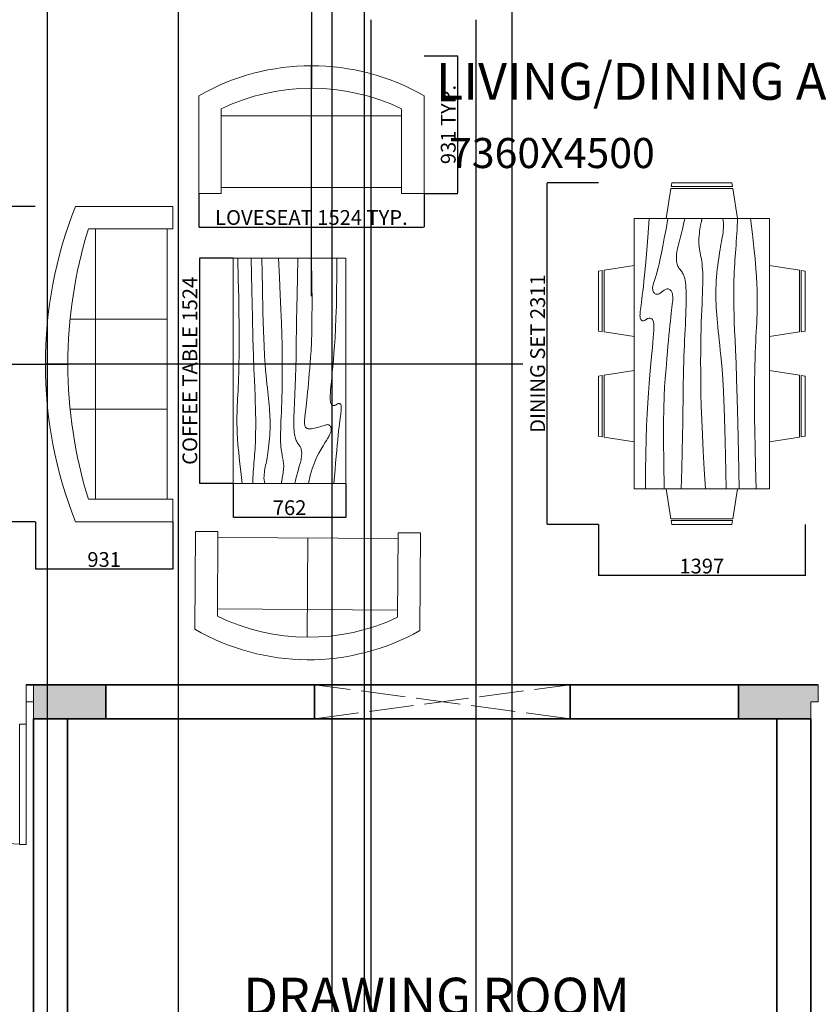
# Model space of a CAD drawing. Units: millimetres. Extents: x -17016 to 4866, y -18325 to 4338.
# Tile 3 of 5: x -8803 to -3399, y -9462 to -2799. Entities that reach past the tile are written whole.
import ezdxf

# ---------------------------------------------------------------- set-up
doc = ezdxf.new("R2010")
doc.units = ezdxf.units.MM
doc.header["$LTSCALE"] = 5
doc.linetypes.add('ACAD_ISO02W100', pattern=[15, 12, -3])
for name, color, linetype, lineweight in [('A-ANNO-DIMS', 2, 'Continuous', 18), ('A-AREA-IDEN', 7, 'Continuous', 25), ('A-COLS', 7, 'Continuous', 35), ('A-COLS-PATT', 252, 'Continuous', 13), ('A-DOOR', 3, 'Continuous', 18), ('A-FURN', 8, 'Continuous', 18), ('A-WALL', 7, 'Continuous', 35), ('A-WALL-OVHD', 8, 'ACAD_ISO02W100', 13)]:
    doc.layers.add(name, color=color, linetype=linetype, lineweight=lineweight)
doc.styles.get("Standard").update_dxf_attribs({"font": 'arial.ttf'})
doc.dimstyles.new('Copy of ISO-25', dxfattribs={"dimtxt": 100, "dimasz": 2.5, "dimexe": 1.25, "dimexo": 0.625, "dimtad": 1, "dimdec": 0, "dimtxsty": 'Standard', "dimcen": 2.5, "dimadec": 0, "dimazin": 0, "dimtfac": 1, "dimtdec": 0, "dimtmove": 0, "dimatfit": 3, "dimfxl": 1, "dimarcsym": 0})

# ---------------------------------------------------------------- blocks, each defined once
blk = doc.blocks.new('Sofa - Roundback 7 ft.')
for p, q in [((-12.00002, -32.4421), (-12.00003, -6.5971)), ((11.99997, -32.4421), (11.99998, -6.5971)), ((-36.000027, -34), (-36.000027, -11.4696)), ((35.99998, -34), (35.99998, -11.4696)), ((-35.999844, -13.3819), (35.9998, -13.3819)), ((-36.000027, -32.4421), (35.99998, -32.4421))]:
    blk.add_line(p, q)
for points in [[(-36.000027, -34), (-42.000027, -34), (-42.000027, -8)], [(41.99998, -8), (41.99998, -34), (35.99998, -34)]]:
    blk.add_lwpolyline(points)
for centre, radius, start, end in [((0, -114.25), 114.25, 68.43141, 111.5686), ((-0.00001, -127.1968), 121.1968, 72.72033, 107.2797)]:
    blk.add_arc(centre, radius, start, end)
blk = doc.blocks.new('Sofa - Roundback Loveseat 5 ft.')
for p, q in [((0, -32.44198), (0, -5.99998)), ((-24, -33.99998), (-24, -11.46958)), ((24.00004, -33.99998), (24.00004, -11.46958)), ((-23.9998, -13.38178), (23.99986, -13.38178)), ((-24, -32.44198), (24.00004, -32.44198))]:
    blk.add_line(p, q)
for points in [[(-24, -33.99998), (-30, -33.99998), (-30, -7.99998)], [(30.00004, -7.99998), (30.00004, -33.99998), (24.00004, -33.99998)]]:
    blk.add_lwpolyline(points)
for centre, radius, start, end in [((0, -60.24998), 60.24998, 60.13715, 119.8628), ((0, -61.38438), 55.38444, 64.32083, 115.6792)]:
    blk.add_arc(centre, radius, start, end)
blk = doc.blocks.new('Table - Rectangular Woodgrain 60 x 30 in.')
for p, q in [((0, 0), (0, -30)), ((60, 0), (0, 0)), ((60, -30), (60, 0)), ((0, -30), (60, -30))]:
    blk.add_line(p, q)
for points in [[(0, -2.4), (4.8155, -2.418), (9.0302, -2.4688), (12.709, -2.5477), (15.9167, -2.65), (18.7181, -2.7711), (21.1781, -2.9063), (23.3616, -3.0508), (25.3333, -3.2), (27.1477, -3.3495), (28.8172, -3.4958), (30.3437, -3.636), (31.7291, -3.7667), (32.9756, -3.8849), (34.0849, -3.9875), (35.059, -4.0714), (35.9, -4.1334), (36.6114, -4.1711), (37.2041, -4.1854), (37.6906, -4.1779), (38.0833, -4.15), (38.3948, -4.1034), (38.6375, -4.0396), (38.8239, -3.9602), (38.9666, -3.8667), (39.0764, -3.7608), (39.1573, -3.6448), (39.2116, -3.521), (39.2416, -3.3917), (39.2498, -3.2593), (39.2385, -3.1261), (39.21, -2.9944), (39.1666, -2.8667), (39.111, -2.7447), (39.0468, -2.6281), (38.978, -2.5163), (38.9083, -2.4083), (38.8418, -2.3035), (38.7823, -2.201), (38.7337, -2.1001), (38.7, -2), (38.6844, -1.9003), (38.6875, -1.8021), (38.7094, -1.707), (38.75, -1.6167), (38.8094, -1.5326), (38.8875, -1.4563), (38.9844, -1.3893), (39.1, -1.3333), (39.2351, -1.2896), (39.3937, -1.2583), (39.5804, -1.2396), (39.8, -1.2333), (40.057, -1.2396), (40.3562, -1.2583), (40.7023, -1.2896), (41.1, -1.3333), (41.5547, -1.3895), (42.0755, -1.4573), (42.6721, -1.5361), (43.3542, -1.625), (44.1316, -1.7233), (45.014, -1.8302), (46.0114, -1.9449), (47.1333, -2.0667), (48.3862, -2.1947), (49.7625, -2.3281), (51.2513, -2.4663), (52.8416, -2.6083), (54.5226, -2.7535), (56.2833, -2.9011), (58.1127, -3.0501), (60, -3.2)], [(0, -9.2), (6.5759, -9.0858), (11.9385, -9.0365), (16.2527, -9.0418), (19.6833, -9.0917), (22.3952, -9.1759), (24.5531, -9.2844), (26.322, -9.4069), (27.8666, -9.5333), (29.3241, -9.6553), (30.7203, -9.7719), (32.0532, -9.8837), (33.3208, -9.9917), (34.5213, -10.0965), (35.6526, -10.199), (36.7128, -10.2999), (37.7, -10.4), (38.6129, -10.4996), (39.4531, -10.5969), (40.223, -10.6895), (40.925, -10.775), (41.5613, -10.8512), (42.1344, -10.9156), (42.6465, -10.966), (43.1, -11), (43.4976, -11.0158), (43.8437, -11.0136), (44.143, -10.9942), (44.4, -10.9583), (44.6195, -10.9069), (44.8062, -10.8406), (44.9648, -10.7603), (45.1, -10.6667), (45.2155, -10.5598), (45.3114, -10.4365), (45.3871, -10.2929), (45.4416, -10.125), (45.4743, -9.929), (45.4844, -9.7011), (45.4709, -9.4371), (45.4333, -9.1333), (45.3716, -8.7883), (45.2896, -8.4104), (45.1919, -8.0107), (45.0833, -7.6), (44.9685, -7.1893), (44.8521, -6.7896), (44.7388, -6.4117), (44.6333, -6.0667), (44.54, -5.7628), (44.4614, -5.4979), (44.4001, -5.2675), (44.3583, -5.0667), (44.3384, -4.8909), (44.3427, -4.7354), (44.3736, -4.5956), (44.4333, -4.4667), (44.5236, -4.3453), (44.6427, -4.2333), (44.7884, -4.1339), (44.9583, -4.05), (45.1501, -3.9849), (45.3614, -3.9417), (45.59, -3.9234), (45.8333, -3.9333), (46.0915, -3.9749), (46.3734, -4.0531), (46.6906, -4.1736), (47.0542, -4.3417), (47.4756, -4.5629), (47.9661, -4.8427), (48.5372, -5.1866), (49.2, -5.6), (49.9676, -6.0844), (50.8594, -6.625), (51.8965, -7.2031), (53.1, -7.8), (54.491, -8.3969), (56.0906, -8.975), (57.9199, -9.5156), (60, -10)], [(0, -12.8), (5.1847, -12.9322), (9.6213, -13.0323), (13.3963, -13.1059), (16.5958, -13.1583), (19.3063, -13.1952), (21.614, -13.2219), (23.6054, -13.2439), (25.3666, -13.2667), (26.9728, -13.2947), (28.4531, -13.3281), (29.8256, -13.3663), (31.1083, -13.4083), (32.3191, -13.4535), (33.476, -13.501), (34.597, -13.5501), (35.7, -13.6), (36.7984, -13.6497), (37.8875, -13.6979), (38.9578, -13.743), (40, -13.7833), (41.0047, -13.8174), (41.9625, -13.8438), (42.864, -13.8607), (43.7, -13.8667), (44.4631, -13.8604), (45.1552, -13.8417), (45.7801, -13.8104), (46.3416, -13.7667), (46.8439, -13.7104), (47.2906, -13.6417), (47.6858, -13.5604), (48.0333, -13.4667), (48.3375, -13.3608), (48.6042, -13.2448), (48.8396, -13.121), (49.05, -12.9917), (49.2417, -12.8593), (49.4208, -12.7261), (49.5937, -12.5944), (49.7667, -12.4667), (49.9452, -12.3451), (50.1323, -12.2313), (50.3303, -12.1268), (50.5416, -12.0333), (50.7686, -11.9524), (51.0135, -11.8854), (51.2788, -11.8341), (51.5666, -11.8), (51.8785, -11.7843), (52.2116, -11.7865), (52.562, -11.8059), (52.926, -11.8417), (53.2998, -11.8931), (53.6795, -11.9594), (54.0614, -12.0397), (54.4416, -12.1333), (54.8223, -12.2401), (55.2293, -12.3625), (55.6942, -12.5037), (56.2489, -12.6667), (56.9251, -12.8547), (57.7545, -13.0708), (58.7689, -13.3182), (60, -13.6)], [(0, -18), (5.124, -17.7273), (9.6609, -17.5057), (13.6705, -17.3303), (17.2125, -17.1958), (20.3467, -17.0973), (23.1328, -17.0297), (25.6307, -16.9878), (27.9, -16.9667), (29.9928, -16.9617), (31.9302, -16.9703), (33.7254, -16.9907), (35.3917, -17.0208), (36.9423, -17.0588), (38.3906, -17.1026), (39.7499, -17.1503), (41.0333, -17.2), (42.2519, -17.2496), (43.4073, -17.2969), (44.4986, -17.3395), (45.525, -17.375), (46.4858, -17.4012), (47.3802, -17.4156), (48.2074, -17.416), (48.9667, -17.4), (49.6583, -17.3662), (50.2872, -17.3167), (50.8595, -17.2547), (51.3812, -17.1833), (51.8584, -17.1057), (52.2971, -17.025), (52.7034, -16.9443), (53.0833, -16.8667), (53.443, -16.7951), (53.789, -16.7313), (54.128, -16.6768), (54.4666, -16.6334), (54.8115, -16.6024), (55.1693, -16.5854), (55.5465, -16.5841), (55.95, -16.6), (56.3828, -16.6337), (56.8346, -16.6823), (57.2915, -16.7418), (57.7396, -16.8084), (58.165, -16.878), (58.5539, -16.9469), (58.8924, -17.0111), (59.1666, -17.0667), (59.3679, -17.1107), (59.5078, -17.1438), (59.6032, -17.1675), (59.6708, -17.1833), (59.7275, -17.193), (59.7901, -17.1979), (59.8753, -17.1998), (60, -17.2)], [(0, -22.4), (8.0098, -22.2501), (14.4094, -22.1011), (19.4168, -21.9535), (23.25, -21.8083), (26.1269, -21.6663), (28.2656, -21.5281), (29.884, -21.3947), (31.2, -21.2667), (32.3967, -21.1448), (33.5172, -21.0292), (34.5697, -20.9198), (35.5625, -20.8167), (36.5037, -20.7198), (37.4015, -20.6292), (38.2642, -20.5448), (39.1, -20.4667), (39.9164, -20.3951), (40.7187, -20.3313), (41.5117, -20.2768), (42.3, -20.2333), (43.0883, -20.2024), (43.8812, -20.1854), (44.6836, -20.1841), (45.5, -20.2), (46.3328, -20.234), (47.1747, -20.2844), (48.0163, -20.3488), (48.8479, -20.425), (49.66, -20.5106), (50.4429, -20.6031), (51.1872, -20.7004), (51.8833, -20.8), (52.5246, -20.8999), (53.1166, -20.9995), (53.6681, -21.0983), (54.1875, -21.1958), (54.6834, -21.2919), (55.1646, -21.3859), (55.6394, -21.4777), (56.1167, -21.5667), (56.6028, -21.6515), (57.0961, -21.7266), (57.5929, -21.7852), (58.0896, -21.8208), (58.5823, -21.8268), (59.0674, -21.7964), (59.5412, -21.723), (60, -21.6)], [(0, -25.2), (8.6355, -25.0504), (15.7026, -24.9031), (21.4049, -24.7606), (25.9458, -24.625), (29.529, -24.4988), (32.3578, -24.3844), (34.6359, -24.284), (36.5667, -24.2), (38.3213, -24.1341), (39.9417, -24.0854), (41.437, -24.0523), (42.8167, -24.0333), (44.0901, -24.0268), (45.2667, -24.0313), (46.3557, -24.0451), (47.3667, -24.0667), (48.309, -24.0947), (49.1928, -24.1287), (50.0284, -24.168), (50.826, -24.2125), (51.5959, -24.2617), (52.3483, -24.3151), (53.0935, -24.3725), (53.8417, -24.4334), (54.6009, -24.497), (55.3699, -24.561), (56.1454, -24.6226), (56.9239, -24.6792), (57.7021, -24.7279), (58.4764, -24.7662), (59.2435, -24.7911), (60, -24.8)], [(0, -28.8), (5.6867, -28.6681), (10.45, -28.5698), (14.407, -28.5012), (17.675, -28.4584), (20.3711, -28.4374), (22.6125, -28.4344), (24.5164, -28.4455), (26.2, -28.4667), (27.762, -28.4947), (29.2276, -28.5281), (30.6033, -28.5663), (31.8958, -28.6084), (33.1118, -28.6535), (34.2578, -28.7011), (35.3405, -28.7501), (36.3666, -28.8), (37.3443, -28.8497), (38.288, -28.8974), (39.2137, -28.9412), (40.1375, -28.9792), (41.0753, -29.0093), (42.0432, -29.0297), (43.0572, -29.0384), (44.1333, -29.0333), (45.2936, -29.0114), (46.5843, -28.9641), (48.0579, -28.8816), (49.7666, -28.7542), (51.7629, -28.5721), (54.0989, -28.3255), (56.8272, -28.0048), (60, -27.6)]]:
    blk.add_lwpolyline(points)
blk = doc.blocks.new('Dining Set - 36 x 72 in.')
for p, q in [((-22, 27.5), (-22.1562, 26.50042)), ((-5.8416, 26.5), (-22.1534, 26.5)), ((-22, 27.5), (-6, 27.5)), ((-5.8437, 26.49966), (-6, 27.5)), ((6, 27.5), (5.8438, 26.50042)), ((22.1584, 26.5), (5.8466, 26.5)), ((6, 27.5), (22, 27.5)), ((22.1563, 26.49966), (22, 27.5)), ((-22.2343, 26.00059), (-23.4847, 17.99762)), ((-22.2304, 26), (-5.7608, 26)), ((-4.5152, 17.99762), (-5.7655, 25.99926)), ((5.7657, 26.00059), (4.5153, 17.99762)), ((5.7696, 26), (22.2392, 26)), ((23.4848, 17.99762), (22.2345, 25.99926)), ((36, 18), (-36, 18)), ((-36, 18), (-36, -18)), ((36, -18), (36, 18)), ((-45.5, 8), (-44.5004, 8.15617)), ((-45.5, 8), (-45.5, -8)), ((-44.5, -8.15843), (-44.5, 8.15338)), ((-44.0006, 8.23428), (-35.9976, 9.48474)), ((-44, 8.23041), (-44, -8.23915)), ((44.0006, 8.23428), (35.9976, 9.48474)), ((44, 8.23041), (44, -8.23915)), ((44.5, -8.15843), (44.5, 8.15338)), ((45.5, 8), (44.5005, 8.15617)), ((45.5, 8), (45.5, -8)), ((-44.4997, -8.15631), (-45.5, -8)), ((-35.9976, -9.48476), (-43.9993, -8.2345)), ((35.9976, -9.48476), (43.9993, -8.2345)), ((44.4997, -8.15631), (45.5, -8)), ((-36, -18), (36, -18)), ((-22.2343, -26.0006), (-23.4847, -17.99762)), ((-4.5152, -17.99762), (-5.7655, -25.99928)), ((5.7657, -26.0006), (4.5153, -17.99762)), ((23.4848, -17.99762), (22.2345, -25.99928)), ((-22.2304, -26), (-5.7608, -26)), ((5.7696, -26), (22.2392, -26)), ((-22, -27.5), (-22.1562, -26.50044)), ((-5.8416, -26.5), (-22.1534, -26.5)), ((-22, -27.5), (-6, -27.5)), ((-5.8437, -26.49967), (-6, -27.5)), ((6, -27.5), (5.8438, -26.50044)), ((22.1584, -26.5), (5.8466, -26.5)), ((6, -27.5), (22, -27.5)), ((22.1563, -26.49967), (22, -27.5))]:
    blk.add_line(p, q)
for points in [[(-36, 15), (-31.1772, 14.97754), (-26.8079, 14.91406), (-22.8538, 14.81543), (-19.276, 14.6875), (-16.0362, 14.53613), (-13.0957, 14.36718), (-10.4159, 14.18652), (-7.9583, 14), (-5.6904, 13.81315), (-3.6035, 13.63021), (-1.6954, 13.45508), (0.0365, 13.29166), (1.5945, 13.14388), (2.9811, 13.01562), (4.1988, 12.9108), (5.25, 12.83333), (6.1393, 12.78613), (6.8802, 12.76823), (7.4883, 12.77767), (7.9792, 12.8125), (8.3685, 12.87077), (8.6719, 12.95052), (8.9049, 13.0498), (9.0833, 13.16666), (9.2205, 13.29899), (9.3216, 13.44401), (9.3895, 13.59879), (9.4271, 13.76041), (9.4373, 13.92594), (9.4232, 14.09245), (9.3875, 14.257), (9.3333, 14.41666), (9.2638, 14.56917), (9.1836, 14.71484), (9.0975, 14.85465), (9.0104, 14.98958), (8.9272, 15.1206), (8.8529, 15.2487), (8.7922, 15.37483), (8.75, 15.5), (8.7305, 15.62467), (8.7344, 15.74739), (8.7617, 15.86621), (8.8125, 15.97916), (8.8867, 16.08431), (8.9844, 16.17968), (9.1055, 16.26334), (9.25, 16.33333), (9.4189, 16.38802), (9.6172, 16.42708), (9.8506, 16.45052), (10.125, 16.45833), (10.4463, 16.45052), (10.8203, 16.42708), (11.2529, 16.38802), (11.75, 16.33333), (12.3184, 16.26318), (12.9694, 16.17838), (13.7151, 16.07991), (14.5677, 15.96875), (15.5395, 15.84586), (16.6426, 15.71224), (17.8893, 15.56884), (19.2917, 15.41666), (20.859, 15.25667), (22.5879, 15.08984), (24.4721, 14.91715), (26.5052, 14.73958), (28.6809, 14.5581), (30.9929, 14.3737), (33.4347, 14.18733), (36, 14)], [(-36, 10), (-28.9766, 10.14274), (-23.1725, 10.20442), (-18.4241, 10.19775), (-14.5677, 10.13541), (-11.4399, 10.03011), (-8.877, 9.89453), (-6.7154, 9.74137), (-4.7917, 9.58333), (-2.9698, 9.43082), (-1.2246, 9.28515), (0.4415, 9.14534), (2.026, 9.01041), (3.5266, 8.87939), (4.9408, 8.7513), (6.266, 8.62516), (7.5, 8.5), (8.6411, 8.37549), (9.6914, 8.2539), (10.6538, 8.13818), (11.5312, 8.03125), (12.3267, 7.93603), (13.043, 7.85547), (13.6831, 7.79248), (14.25, 7.75), (14.7471, 7.7303), (15.1797, 7.73307), (15.5537, 7.75732), (15.875, 7.80208), (16.1494, 7.86637), (16.3828, 7.94922), (16.5811, 8.04964), (16.75, 8.16666), (16.8944, 8.29915), (17.0143, 8.44531), (17.1089, 8.60319), (17.1771, 8.77083), (17.218, 8.94629), (17.2305, 9.1276), (17.2137, 9.31282), (17.1667, 9.5), (17.0895, 9.6875), (16.987, 9.875), (16.8649, 10.0625), (16.7292, 10.25), (16.5856, 10.4375), (16.4401, 10.625), (16.2985, 10.8125), (16.1667, 11), (16.05, 11.18733), (15.9518, 11.3737), (15.8752, 11.5581), (15.8229, 11.73958), (15.798, 11.91715), (15.8034, 12.08984), (15.842, 12.25667), (15.9167, 12.41666), (16.0295, 12.56836), (16.1784, 12.70833), (16.3605, 12.83268), (16.5729, 12.9375), (16.8127, 13.01888), (17.0768, 13.07291), (17.3625, 13.0957), (17.6667, 13.08333), (17.9894, 13.03312), (18.3418, 12.94726), (18.7382, 12.82918), (19.1927, 12.68229), (19.7195, 12.51001), (20.3327, 12.31575), (21.0465, 12.10294), (21.875, 11.875), (22.8357, 11.63354), (23.959, 11.37304), (25.2786, 11.08618), (26.8282, 10.76562), (28.6414, 10.40405), (30.752, 9.99414), (33.1936, 9.52856), (36, 9)], [(-36, 5.5), (-30.7157, 5.3348), (-26.069, 5.20963), (-21.9946, 5.11767), (-18.4271, 5.05208), (-15.3009, 5.00602), (-12.5508, 4.97265), (-10.1112, 4.94515), (-7.9167, 4.91666), (-5.909, 4.88167), (-4.0586, 4.83984), (-2.3429, 4.79215), (-0.7396, 4.73958), (0.7739, 4.6831), (2.22, 4.6237), (3.6213, 4.56233), (5, 4.5), (6.373, 4.43782), (7.7344, 4.3776), (9.0723, 4.32129), (10.375, 4.27083), (11.6309, 4.22819), (12.8281, 4.19531), (13.9551, 4.17415), (15, 4.16666), (15.954, 4.17448), (16.819, 4.19791), (17.6001, 4.23698), (18.3021, 4.29166), (18.9299, 4.36198), (19.4883, 4.44791), (19.9823, 4.54948), (20.4167, 4.66666), (20.7969, 4.79899), (21.1302, 4.94401), (21.4245, 5.09879), (21.6875, 5.26041), (21.9271, 5.42594), (22.1511, 5.59245), (22.3672, 5.757), (22.5834, 5.91666), (22.8065, 6.06868), (23.0404, 6.21093), (23.2879, 6.34147), (23.5521, 6.45833), (23.8358, 6.55957), (24.142, 6.64323), (24.4735, 6.70735), (24.8334, 6.75), (25.2235, 6.76969), (25.642, 6.76692), (26.0858, 6.74267), (26.5521, 6.69791), (27.0379, 6.63362), (27.5404, 6.55078), (28.0565, 6.45036), (28.5834, 6.33333), (29.1242, 6.19987), (29.7071, 6.04687), (30.3661, 5.87044), (31.1354, 5.66666), (32.0493, 5.43164), (33.142, 5.16146), (34.4475, 4.85221), (36, 4.5)], [(-36, -1), (-30.7915, -0.6591), (-26.0195, -0.38216), (-21.6519, -0.16284), (-17.6563, 0.00521), (-14.0005, 0.12833), (-10.6523, 0.21289), (-7.5796, 0.26522), (-4.75, 0.29166), (-2.134, 0.29793), (0.2878, 0.28711), (2.5317, 0.26163), (4.6146, 0.22396), (6.5529, 0.17651), (8.3633, 0.12174), (10.0623, 0.06209), (11.6667, 0), (13.1899, -0.06201), (14.6341, -0.1211), (15.9982, -0.17432), (17.2813, -0.21875), (18.4823, -0.25147), (19.6003, -0.26953), (20.6343, -0.27002), (21.5834, -0.25), (22.4481, -0.20768), (23.2357, -0.14584), (23.9549, -0.06836), (24.6146, 0.02083), (25.2235, 0.11784), (25.7904, 0.21875), (26.3241, 0.31966), (26.8334, 0.41666), (27.3265, 0.50618), (27.8099, 0.58593), (28.2894, 0.65397), (28.7709, 0.70833), (29.2601, 0.74707), (29.763, 0.76823), (30.2855, 0.76985), (30.8334, 0.75), (31.4088, 0.70784), (31.9994, 0.64713), (32.589, 0.57275), (33.1615, 0.48958), (33.7008, 0.4025), (34.1908, 0.3164), (34.6153, 0.23616), (34.9584, 0.16666), (35.2099, 0.11165), (35.3848, 0.07031), (35.504, 0.04069), (35.5886, 0.02083), (35.6594, 0.00879), (35.7377, 0.0026), (35.8442, 0.00032), (36, 0)], [(-36, -6.5), (-27.1843, -6.31267), (-20.084, -6.1263), (-14.469, -5.9419), (-10.1094, -5.76042), (-6.7752, -5.58285), (-4.2363, -5.41016), (-2.2629, -5.24333), (-0.625, -5.08334), (0.8708, -4.93099), (2.2715, -4.78646), (3.5872, -4.64974), (4.8281, -4.52084), (6.0046, -4.39974), (7.127, -4.28646), (8.2053, -4.18099), (9.25, -4.08334), (10.2705, -3.99382), (11.2734, -3.91407), (12.2647, -3.84603), (13.25, -3.79167), (14.2354, -3.75293), (15.2266, -3.73177), (16.2295, -3.73015), (17.25, -3.75), (18.2912, -3.79248), (19.3451, -3.85547), (20.4009, -3.93604), (21.4479, -4.03125), (22.4754, -4.13819), (23.4727, -4.25391), (24.4289, -4.37549), (25.3334, -4.5), (26.1785, -4.62492), (26.9694, -4.74935), (27.7145, -4.87281), (28.4219, -4.99479), (29.1, -5.11483), (29.7572, -5.23242), (30.4016, -5.34709), (31.0417, -5.45834), (31.6837, -5.56437), (32.3262, -5.65821), (32.9658, -5.73153), (33.599, -5.77604), (34.2224, -5.78345), (34.8327, -5.74545), (35.4264, -5.65373), (36, -5.5)], [(-36, -10), (-26.4022, -9.81299), (-18.4675, -9.62891), (-11.9839, -9.45069), (-6.7396, -9.28125), (-2.5226, -9.12354), (0.8789, -8.98047), (3.6769, -8.85498), (6.0833, -8.75), (8.2767, -8.66765), (10.3021, -8.60677), (12.1712, -8.56543), (13.8958, -8.54167), (15.4876, -8.53353), (16.9583, -8.53907), (18.3197, -8.55632), (19.5834, -8.58334), (20.7616, -8.61841), (21.8685, -8.66081), (22.9188, -8.71004), (23.9271, -8.76563), (24.9081, -8.82707), (25.8763, -8.89388), (26.8465, -8.96558), (27.8334, -9.04167), (28.8474, -9.12118), (29.8828, -9.20117), (30.93, -9.27824), (31.9792, -9.34896), (33.0205, -9.40991), (34.0443, -9.45768), (35.0407, -9.48885), (36, -9.5)], [(-36, -14.5), (-30.0881, -14.33513), (-25.0332, -14.21224), (-20.7312, -14.12647), (-17.0781, -14.07292), (-13.97, -14.04671), (-11.3027, -14.04297), (-8.9724, -14.05681), (-6.875, -14.08334), (-4.9224, -14.11833), (-3.0905, -14.16016), (-1.3709, -14.20785), (0.2448, -14.26042), (1.7647, -14.3169), (3.1973, -14.3763), (4.5507, -14.43767), (5.8333, -14.5), (7.0554, -14.5621), (8.235, -14.62175), (9.3922, -14.67652), (10.5469, -14.72396), (11.7192, -14.76164), (12.929, -14.78711), (14.1965, -14.79794), (15.5417, -14.79167), (16.9933, -14.76424), (18.6152, -14.70508), (20.4804, -14.60197), (22.6615, -14.44271), (25.2312, -14.21509), (28.2624, -13.9069), (31.8277, -13.50594), (36, -13)]]:
    blk.add_lwpolyline(points)
blk = doc.blocks.new('*U2')
for p, q in [((0, 0), (0, -6)), ((32, 0), (32, -6))]:
    blk.add_line(p, q)
blk.add_lwpolyline([(0, 0), (0, 32), (1.75, 32), (1.75, 0)], close=True)
blk.add_arc((0, 0), 32, 0, 90)
blk = doc.blocks.new('*D32')
at = {"layer": 'A-ANNO-DIMS', "color": 0, "lineweight": -2, "ltscale": 5, "transparency": 16777216}
for p, q in [((-7591, -3974.9), (-7591, -4204.1)), ((-6067, -3974.9), (-6067, -4204.1)), ((-7588.5, -4202.9), (-6069.5, -4202.9))]:
    blk.add_line(p, q, dxfattribs=at)
at = {"layer": 'A-ANNO-DIMS', "color": 0, "ltscale": 5, "transparency": 16777216}
for points in [[(-7588.5, -4202.5), (-7588.5, -4203.3), (-7591, -4202.9)], [(-6069.5, -4202.5), (-6069.5, -4203.3), (-6067, -4202.9)]]:
    blk.add_solid(points, dxfattribs=at)
at = {"layer": 'Defpoints', "color": 0, "ltscale": 5, "transparency": 16777216}
for p in [(-7591, -3974.3), (-6067, -3974.3), (-6067, -4202.9)]:
    blk.add_point(p, dxfattribs=at)
at = {"layer": 'A-ANNO-DIMS', "color": 0, "ltscale": 5, "transparency": 16777216, "insert": (-6829, -4150.5), "char_height": 100, "attachment_point": 5}
blk.add_mtext('LOVESEAT 1524 TYP.', dxfattribs=at)
blk = doc.blocks.new('*D33')
at = {"layer": 'A-ANNO-DIMS', "color": 0, "lineweight": -2, "ltscale": 5, "transparency": 16777216}
for p, q in [((-6066.4, -3043), (-5837.1, -3043)), ((-5838.4, -3971.8), (-5838.4, -3045.5)), ((-6066.4, -3974.3), (-5837.1, -3974.3))]:
    blk.add_line(p, q, dxfattribs=at)
at = {"layer": 'A-ANNO-DIMS', "color": 0, "ltscale": 5, "transparency": 16777216}
for points in [[(-5838.8, -3045.5), (-5838, -3045.5), (-5838.4, -3043)], [(-5838.8, -3971.8), (-5838, -3971.8), (-5838.4, -3974.3)]]:
    blk.add_solid(points, dxfattribs=at)
at = {"layer": 'Defpoints', "color": 0, "ltscale": 5, "transparency": 16777216}
for p in [(-6067, -3043), (-5838.4, -3043), (-6067, -3974.3)]:
    blk.add_point(p, dxfattribs=at)
at = {"layer": 'A-ANNO-DIMS', "color": 0, "ltscale": 5, "transparency": 16777216, "insert": (-5890.1, -3508.6), "char_height": 100, "attachment_point": 5, "rotation": 90}
blk.add_mtext('931 TYP.', dxfattribs=at)
blk = doc.blocks.new('*D36')
at = {"layer": 'A-ANNO-DIMS', "color": 0, "lineweight": -2, "ltscale": 5, "transparency": 16777216}
for p, q in [((-8697.6, -4062.9), (-9018.2, -4062.9)), ((-9017, -6194), (-9017, -4065.4)), ((-8697.6, -6196.5), (-9018.2, -6196.5))]:
    blk.add_line(p, q, dxfattribs=at)
at = {"layer": 'A-ANNO-DIMS', "color": 0, "ltscale": 5, "transparency": 16777216}
for points in [[(-9017.4, -4065.4), (-9016.6, -4065.4), (-9017, -4062.9)], [(-9017.4, -6194), (-9016.6, -6194), (-9017, -6196.5)]]:
    blk.add_solid(points, dxfattribs=at)
at = {"layer": 'Defpoints', "color": 0, "ltscale": 5, "transparency": 16777216}
for p in [(-9017, -4062.9), (-8696.9, -4062.9), (-8696.9, -6196.5)]:
    blk.add_point(p, dxfattribs=at)
at = {"layer": 'A-ANNO-DIMS', "color": 0, "ltscale": 5, "transparency": 16777216, "insert": (-9069.4, -5129.7), "char_height": 100, "attachment_point": 5, "rotation": 90}
blk.add_mtext('SOFA 2134', dxfattribs=at)
blk = doc.blocks.new('*D37')
at = {"layer": 'A-ANNO-DIMS', "color": 0, "lineweight": -2, "ltscale": 5, "transparency": 16777216}
for p, q in [((-8696.9, -6197.1), (-8696.9, -6517.8)), ((-7765.6, -6197.1), (-7765.6, -6517.8)), ((-7768.1, -6516.5), (-8694.4, -6516.5))]:
    blk.add_line(p, q, dxfattribs=at)
at = {"layer": 'A-ANNO-DIMS', "color": 0, "ltscale": 5, "transparency": 16777216}
for points in [[(-8694.4, -6516.1), (-8694.4, -6516.9), (-8696.9, -6516.5)], [(-7768.1, -6516.1), (-7768.1, -6516.9), (-7765.6, -6516.5)]]:
    blk.add_solid(points, dxfattribs=at)
at = {"layer": 'Defpoints', "color": 0, "ltscale": 5, "transparency": 16777216}
for p in [(-8696.9, -6196.5), (-7765.6, -6196.5), (-8696.9, -6516.5)]:
    blk.add_point(p, dxfattribs=at)
at = {"layer": 'A-ANNO-DIMS', "color": 0, "ltscale": 5, "transparency": 16777216, "insert": (-8231.3, -6464.8), "char_height": 100, "attachment_point": 5, "rotation": 359.99998}
blk.add_mtext('931', dxfattribs=at)
blk = doc.blocks.new('*D38')
at = {"layer": 'A-ANNO-DIMS', "color": 0, "lineweight": -2, "ltscale": 5, "transparency": 16777216}
for p, q in [((-7358, -4413.1), (-7587.2, -4413.1)), ((-7586, -4415.6), (-7586, -5934.6)), ((-7358, -5937.1), (-7587.2, -5937.1))]:
    blk.add_line(p, q, dxfattribs=at)
at = {"layer": 'A-ANNO-DIMS', "color": 0, "ltscale": 5, "transparency": 16777216}
for points in [[(-7586.4, -4415.6), (-7585.6, -4415.6), (-7586, -4413.1)], [(-7586.4, -5934.6), (-7585.6, -5934.6), (-7586, -5937.1)]]:
    blk.add_solid(points, dxfattribs=at)
at = {"layer": 'Defpoints', "color": 0, "ltscale": 5, "transparency": 16777216}
for p in [(-7357.4, -4413.1), (-7586, -5937.1), (-7357.4, -5937.1)]:
    blk.add_point(p, dxfattribs=at)
at = {"layer": 'A-ANNO-DIMS', "color": 0, "ltscale": 5, "transparency": 16777216, "insert": (-7638.4, -5175.1), "char_height": 100, "attachment_point": 5, "rotation": 90}
blk.add_mtext('COFFEE TABLE 1524', dxfattribs=at)
blk = doc.blocks.new('*D39')
at = {"layer": 'A-ANNO-DIMS', "color": 0, "lineweight": -2, "ltscale": 5, "transparency": 16777216}
for p, q in [((-7357.4, -5937.8), (-7357.4, -6167)), ((-6595.4, -5937.8), (-6595.4, -6167)), ((-7354.9, -6165.7), (-6597.9, -6165.7))]:
    blk.add_line(p, q, dxfattribs=at)
at = {"layer": 'A-ANNO-DIMS', "color": 0, "ltscale": 5, "transparency": 16777216}
for points in [[(-7354.9, -6165.3), (-7354.9, -6166.1), (-7357.4, -6165.7)], [(-6597.9, -6165.3), (-6597.9, -6166.1), (-6595.4, -6165.7)]]:
    blk.add_solid(points, dxfattribs=at)
at = {"layer": 'Defpoints', "color": 0, "ltscale": 5, "transparency": 16777216}
for p in [(-7357.4, -5937.1), (-6595.4, -5937.1), (-6595.4, -6165.7)]:
    blk.add_point(p, dxfattribs=at)
at = {"layer": 'A-ANNO-DIMS', "color": 0, "ltscale": 5, "transparency": 16777216, "insert": (-6976.4, -6114), "char_height": 100, "attachment_point": 5}
blk.add_mtext('762', dxfattribs=at)
blk = doc.blocks.new('*D40')
at = {"layer": 'A-ANNO-DIMS', "color": 0, "lineweight": -2, "ltscale": 5, "transparency": 16777216}
for p, q in [((-4886.8, -3902.9), (-5234.1, -3902.9)), ((-5232.8, -6211.8), (-5232.8, -3905.4)), ((-4886.8, -6214.3), (-5234.1, -6214.3))]:
    blk.add_line(p, q, dxfattribs=at)
at = {"layer": 'A-ANNO-DIMS', "color": 0, "ltscale": 5, "transparency": 16777216}
for points in [[(-5233.3, -3905.4), (-5232.4, -3905.4), (-5232.8, -3902.9)], [(-5233.3, -6211.8), (-5232.4, -6211.8), (-5232.8, -6214.3)]]:
    blk.add_solid(points, dxfattribs=at)
at = {"layer": 'Defpoints', "color": 0, "ltscale": 5, "transparency": 16777216}
for p in [(-5232.8, -3902.9), (-4886.1, -3902.9), (-4886.1, -6214.3)]:
    blk.add_point(p, dxfattribs=at)
at = {"layer": 'A-ANNO-DIMS', "color": 0, "ltscale": 5, "transparency": 16777216, "insert": (-5285.2, -5058.6), "char_height": 100, "attachment_point": 5, "rotation": 90}
blk.add_mtext('DINING SET 2311', dxfattribs=at)
blk = doc.blocks.new('*D41')
at = {"layer": 'A-ANNO-DIMS', "color": 0, "lineweight": -2, "ltscale": 5, "transparency": 16777216}
for p, q in [((-4886.1, -6214.9), (-4886.1, -6562.3)), ((-3489.1, -6214.9), (-3489.1, -6562.3)), ((-3491.6, -6561), (-4883.6, -6561))]:
    blk.add_line(p, q, dxfattribs=at)
at = {"layer": 'A-ANNO-DIMS', "color": 0, "ltscale": 5, "transparency": 16777216}
for points in [[(-4883.6, -6560.6), (-4883.6, -6561.4), (-4886.1, -6561)], [(-3491.6, -6560.6), (-3491.6, -6561.4), (-3489.1, -6561)]]:
    blk.add_solid(points, dxfattribs=at)
at = {"layer": 'Defpoints', "color": 0, "ltscale": 5, "transparency": 16777216}
for p in [(-4886.1, -6214.3), (-3489.1, -6214.3), (-4886.1, -6561)]:
    blk.add_point(p, dxfattribs=at)
at = {"layer": 'A-ANNO-DIMS', "color": 0, "ltscale": 5, "transparency": 16777216, "insert": (-4187.6, -6509.3), "char_height": 100, "attachment_point": 5}
blk.add_mtext('1397', dxfattribs=at)
blk = doc.blocks.new('*D51')
at = {"layer": 'A-ANNO-DIMS', "color": 0, "lineweight": -2, "ltscale": 5, "transparency": 16777216}
for p, q in [((-6427.6, -2799.7), (-6427.6, -18311.8)), ((-5716.4, -2799.7), (-5716.4, -18311.8)), ((-6425.1, -18310.6), (-5718.9, -18310.6))]:
    blk.add_line(p, q, dxfattribs=at)
at = {"layer": 'A-ANNO-DIMS', "color": 0, "ltscale": 5, "transparency": 16777216}
for points in [[(-6425.1, -18310.2), (-6425.1, -18311), (-6427.6, -18310.6)], [(-5718.9, -18310.2), (-5718.9, -18311), (-5716.4, -18310.6)]]:
    blk.add_solid(points, dxfattribs=at)
at = {"layer": 'Defpoints', "color": 0, "ltscale": 5, "transparency": 16777216}
for p in [(-6427.6, -2799.1), (-5716.4, -2799.1), (-5716.4, -18310.6)]:
    blk.add_point(p, dxfattribs=at)
at = {"layer": 'A-ANNO-DIMS', "color": 0, "ltscale": 5, "transparency": 16777216, "insert": (-6072, -18259.8), "char_height": 100, "attachment_point": 5}
blk.add_mtext('711.2', dxfattribs=at)
blk = doc.blocks.new('*D53')
at = {"layer": 'A-ANNO-DIMS', "color": 0, "lineweight": -2, "ltscale": 5, "transparency": 16777216}
for p, q in [((-6688.8, -11408.5), (-6688.8, 4221.9)), ((-6686.3, 4220.6), (-5472.1, 4220.6)), ((-5469.6, -11408.5), (-5469.6, 4221.9))]:
    blk.add_line(p, q, dxfattribs=at)
at = {"layer": 'A-ANNO-DIMS', "color": 0, "ltscale": 5, "transparency": 16777216}
for points in [[(-6686.3, 4221.1), (-6686.3, 4220.2), (-6688.8, 4220.6)], [(-5472.1, 4221.1), (-5472.1, 4220.2), (-5469.6, 4220.6)]]:
    blk.add_solid(points, dxfattribs=at)
at = {"layer": 'Defpoints', "color": 0, "ltscale": 5, "transparency": 16777216}
for p in [(-5469.6, 4220.6), (-6688.8, -11409.1), (-5469.6, -11409.1)]:
    blk.add_point(p, dxfattribs=at)
at = {"layer": 'A-ANNO-DIMS', "color": 0, "ltscale": 5, "transparency": 16777216, "insert": (-6079.2, 4272.3), "char_height": 100, "attachment_point": 5}
blk.add_mtext('1219.2', dxfattribs=at)
blk = doc.blocks.new('*D54')
at = {"layer": 'A-ANNO-DIMS', "color": 0, "lineweight": -2, "ltscale": 5, "transparency": 16777216}
for p, q in [((-7729.9, 1140.6), (-7729.9, -18311.8)), ((-6472.1, 1140.6), (-6472.1, -18311.8)), ((-7727.4, -18310.6), (-6474.6, -18310.6))]:
    blk.add_line(p, q, dxfattribs=at)
at = {"layer": 'A-ANNO-DIMS', "color": 0, "ltscale": 5, "transparency": 16777216}
for points in [[(-7727.4, -18310.2), (-7727.4, -18311), (-7729.9, -18310.6)], [(-6474.6, -18310.2), (-6474.6, -18311), (-6472.1, -18310.6)]]:
    blk.add_solid(points, dxfattribs=at)
at = {"layer": 'Defpoints', "color": 0, "ltscale": 5, "transparency": 16777216}
for p in [(-7729.9, 1141.2), (-6472.1, 1141.2), (-6472.1, -18310.6)]:
    blk.add_point(p, dxfattribs=at)
at = {"layer": 'A-ANNO-DIMS', "color": 0, "ltscale": 5, "transparency": 16777216, "insert": (-7101, -18258.9), "char_height": 100, "attachment_point": 5}
blk.add_mtext('1257.7', dxfattribs=at)
blk = doc.blocks.new('*D56')
at = {"layer": 'A-ANNO-DIMS', "color": 0, "lineweight": -2, "ltscale": 5, "transparency": 16777216}
for p, q in [((-8616.4, -2525.4), (-8616.4, -18311.8)), ((-7729.9, -2525.4), (-7729.9, -18311.8)), ((-8613.9, -18310.6), (-7732.4, -18310.6))]:
    blk.add_line(p, q, dxfattribs=at)
at = {"layer": 'A-ANNO-DIMS', "color": 0, "ltscale": 5, "transparency": 16777216}
for points in [[(-8613.9, -18310.2), (-8613.9, -18311), (-8616.4, -18310.6)], [(-7732.4, -18310.2), (-7732.4, -18311), (-7729.9, -18310.6)]]:
    blk.add_solid(points, dxfattribs=at)
at = {"layer": 'Defpoints', "color": 0, "ltscale": 5, "transparency": 16777216}
for p in [(-8616.4, -2524.7), (-7729.9, -2524.7), (-7729.9, -18310.6)]:
    blk.add_point(p, dxfattribs=at)
at = {"layer": 'A-ANNO-DIMS', "color": 0, "ltscale": 5, "transparency": 16777216, "insert": (-8173.1, -18258.9), "char_height": 100, "attachment_point": 5}
blk.add_mtext('886.5', dxfattribs=at)
blk = doc.blocks.new('*D57')
at = {"layer": 'A-ANNO-DIMS', "color": 0, "lineweight": -2, "ltscale": 5, "transparency": 16777216}
for p, q in [((-10579.7, -5129.7), (-8479.3, -5129.7)), ((-5398.4, -5129.7), (-8476.8, -5129.7))]:
    blk.add_line(p, q, dxfattribs=at)
at = {"layer": 'A-ANNO-DIMS', "color": 0, "ltscale": 5, "transparency": 16777216}
blk.add_solid([(-8479.3, -5129.2), (-8479.3, -5130.1), (-8476.8, -5129.7)], dxfattribs=at)
at = {"layer": 'Defpoints', "color": 0, "ltscale": 5, "transparency": 16777216}
for p in [(-8476.8, -5129.7), (-5398.4, -5129.7)]:
    blk.add_point(p, dxfattribs=at)
at = {"layer": 'A-ANNO-DIMS', "color": 0, "ltscale": 5, "transparency": 16777216, "insert": (-10323.8, -5077.9), "char_height": 100, "attachment_point": 5}
blk.add_mtext('R3078.4', dxfattribs=at)
blk = doc.blocks.new('*D58')
at = {"layer": 'A-ANNO-DIMS', "color": 0, "lineweight": -2, "ltscale": 5, "transparency": 16777216}
for p, q in [((-10567.7, -5129.7), (-8631.7, -5129.7)), ((-5727.3, -5129.7), (-8629.2, -5129.7))]:
    blk.add_line(p, q, dxfattribs=at)
at = {"layer": 'A-ANNO-DIMS', "color": 0, "ltscale": 5, "transparency": 16777216}
blk.add_solid([(-8631.7, -5129.2), (-8631.7, -5130.1), (-8629.2, -5129.7)], dxfattribs=at)
at = {"layer": 'Defpoints', "color": 0, "ltscale": 5, "transparency": 16777216}
for p in [(-8629.2, -5129.7), (-5727.3, -5129.7)]:
    blk.add_point(p, dxfattribs=at)
at = {"layer": 'A-ANNO-DIMS', "color": 0, "ltscale": 5, "transparency": 16777216, "insert": (-10370.4, -5078), "char_height": 100, "attachment_point": 5}
blk.add_mtext('R2902', dxfattribs=at)
blk = doc.blocks.new('*D59')
at = {"layer": 'A-ANNO-DIMS', "color": 0, "lineweight": -2, "ltscale": 5, "transparency": 16777216}
for p, q in [((-6829, -1936.4), (-6829, -3108.2)), ((-6829, -4641), (-6829, -3110.7))]:
    blk.add_line(p, q, dxfattribs=at)
at = {"layer": 'A-ANNO-DIMS', "color": 0, "ltscale": 5, "transparency": 16777216}
blk.add_solid([(-6829.4, -3108.2), (-6828.6, -3108.2), (-6829, -3110.7)], dxfattribs=at)
at = {"layer": 'Defpoints', "color": 0, "ltscale": 5, "transparency": 16777216}
for p in [(-6829, -3110.7), (-6829, -4641)]:
    blk.add_point(p, dxfattribs=at)
at = {"layer": 'A-ANNO-DIMS', "color": 0, "ltscale": 5, "transparency": 16777216, "insert": (-6880.7, -2192.5), "char_height": 100, "attachment_point": 5, "rotation": 90}
blk.add_mtext('R1530.3', dxfattribs=at)
blk = doc.blocks.new('*D60')
at = {"layer": 'A-ANNO-DIMS', "color": 0, "lineweight": -2, "ltscale": 5, "transparency": 16777216}
for p, q in [((-6829, -2162.9), (-6829, -3260.6)), ((-6829, -4669.8), (-6829, -3263.1))]:
    blk.add_line(p, q, dxfattribs=at)
at = {"layer": 'A-ANNO-DIMS', "color": 0, "ltscale": 5, "transparency": 16777216}
blk.add_solid([(-6829.4, -3260.6), (-6828.6, -3260.6), (-6829, -3263.1)], dxfattribs=at)
at = {"layer": 'Defpoints', "color": 0, "ltscale": 5, "transparency": 16777216}
for p in [(-6829, -3263.1), (-6829, -4669.8)]:
    blk.add_point(p, dxfattribs=at)
at = {"layer": 'A-ANNO-DIMS', "color": 0, "ltscale": 5, "transparency": 16777216, "insert": (-6880.7, -2419), "char_height": 100, "attachment_point": 5, "rotation": 90}
blk.add_mtext('R1406.8', dxfattribs=at)

msp = doc.modelspace()

# ---------------------------------------------------------------- hatches: boundary and pattern name
at = {"layer": 'A-COLS-PATT', "ltscale": 5}
h = msp.add_hatch(color=256, dxfattribs=at)
h.dxf.hatch_style = 1
h.paths.add_polyline_path([(980.82, -7299.11), (490.82, -7299.11), (490.82, -7529.11), (980.82, -7529.11)])
h.paths.add_polyline_path([(-3449.18, -7414.11), (-3399.18, -7414.11), (-3399.18, -7299.11), (-3939.18, -7299.11), (-3939.18, -7529.11), (-3449.18, -7529.11)])
h.paths.add_polyline_path([(-8219.18, -7299.11), (-8709.18, -7299.11), (-8709.18, -7529.11), (-8219.18, -7529.11)])
h.paths.add_polyline_path([(-12649.22, -7299.11), (-13139.18, -7299.11), (-13139.18, -7529.11), (-12649.22, -7529.11)])

# ---------------------------------------------------------------- linework, layer by layer
at = {"layer": 'A-COLS', "ltscale": 5}
for p, q in [((-8219.18, -7529.11), (-8219.18, -7299.11)), ((-3939.18, -7529.11), (-3939.18, -7299.11))]:
    msp.add_line(p, q, dxfattribs=at)
at = {"layer": 'A-DOOR'}
for p, q in [((-8759.18, -7414.11), (-8759.18, -7299.11)), ((-8709.18, -7529.11), (-8709.18, -7299.11)), ((-3399.18, -7414.11), (-3399.18, -7299.11)), ((-8709.18, -7414.11), (-8759.18, -7414.11)), ((-3449.18, -7529.11), (-3449.18, -7414.11)), ((-3399.18, -7414.11), (-3449.18, -7414.11))]:
    msp.add_line(p, q, dxfattribs=at)
at = {"layer": 'A-WALL'}
for p, q in [((-3399.18, -7299.11), (-8759.18, -7299.11)), ((-8709.18, -7529.11), (-8709.18, -12909.11)), ((-3449.18, -7529.11), (-8709.18, -7529.11)), ((-8479.18, -7529.11), (-8479.18, -12909.11)), ((-3679.18, -7529.11), (-3679.18, -12909.11)), ((-3449.18, -7529.11), (-3449.18, -9409.11)), ((-3449.18, -9409.11), (-3449.18, -12909.11))]:
    msp.add_line(p, q, dxfattribs=at)
at = {"layer": 'A-WALL', "ltscale": 5}
for p, q in [((-6807.37, -7529.11), (-6807.37, -7299.11)), ((-5079.18, -7529.11), (-5079.18, -7299.11))]:
    msp.add_line(p, q, dxfattribs=at)
at = {"layer": 'A-WALL-OVHD', "ltscale": 5}
for p, q in [((-6807.37, -7529.11), (-5079.18, -7299.11)), ((-5079.18, -7529.11), (-6807.37, -7299.11))]:
    msp.add_line(p, q, dxfattribs=at)

# ---------------------------------------------------------------- block references
at = {"layer": 'A-DOOR', "xscale": 25.4, "yscale": 25.4, "zscale": 25.4, "rotation": 180}
msp.add_blockref('*U2', (-8759.18, -7566.51), dxfattribs=at)
at = {"layer": 'A-FURN', "xscale": 25.4, "yscale": 25.4, "zscale": 25.4}
msp.add_blockref('Sofa - Roundback Loveseat 5 ft.', (-6828.98, -3110.69), dxfattribs=at)
at = {"layer": 'A-FURN', "zscale": 25.4}
for name, p, xscale, yscale, rotation in [('Dining Set - 36 x 72 in.', (-4187.63, -5058.61), 25.4, 25.4, 90), ('Sofa - Roundback 7 ft.', (-8629.21, -5129.66), 25.4, 25.4, 89.99997936313684), ('Table - Rectangular Woodgrain 60 x 30 in.', (-6595.39, -4413.13), 25.4, 25.4, 270), ('Sofa - Roundback Loveseat 5 ft.', (-6857.51, -7130.29), -25.39999999999999, 25.39999999999999, 179.64900727918)]:
    msp.add_blockref(name, p, dxfattribs=dict(at, xscale=xscale, yscale=yscale, rotation=rotation))

# ---------------------------------------------------------------- texts
at = {"layer": 'A-AREA-IDEN', "ltscale": 5}
for s, height, p in [('LIVING/DINING AREA', 250, (-5986.71, -3341.18)), ('7360X4500', 203.546, (-5897.56, -3803.15)), ('DRAWING ROOM', 250, (-7289.61, -9531.88))]:
    msp.add_text(s, height=height, dxfattribs=at).set_placement(p)

# ---------------------------------------------------------------- dimensions: what is measured, and where the dimension line sits
at = {"layer": 'A-ANNO-DIMS', "ltscale": 5}
for base, p1, p2, override, picture, middle in [((-5469.58, 4220.64), (-6688.77, -11409.11), (-5469.58, -11409.11), {"dimdec": 1, "dimlfac": 1, "dimrnd": 0, "dimzin": 0, "dimdsep": 46, "dimlunit": 2}, '*D53', (-6079.18, 4272.32)), ((-6472.15, -18310.58), (-7729.85, 1141.22), (-6472.15, 1141.22), {"dimdec": 1, "dimlfac": 1, "dimrnd": 0, "dimzin": 0, "dimdsep": 46, "dimlunit": 2}, '*D54', (-7101, -18258.9)), ((-7729.85, -18310.58), (-8616.38, -2524.75), (-7729.85, -2524.75), {"dimdec": 1, "dimlfac": 1, "dimrnd": 0, "dimzin": 0, "dimdsep": 46, "dimlunit": 2}, '*D56', (-8173.11, -18258.9)), ((-5716.38, -18310.58), (-6427.58, -2799.11), (-5716.38, -2799.11), {"dimdec": 1, "dimlfac": 1, "dimrnd": 0, "dimzin": 0, "dimdsep": 46, "dimlunit": 2}, '*D51', (-6071.98, -18259.75)), ((-6595.39, -6165.73), (-7357.39, -5937.13), (-6595.39, -5937.13), {"dimdec": 0, "dimlfac": 1, "dimrnd": 0, "dimzin": 0, "dimdsep": 46, "dimlunit": 2}, '*D39', (-6976.39, -6114.05))]:
    dim = msp.add_linear_dim(base=base, p1=p1, p2=p2, dimstyle='Copy of ISO-25', override=override, dxfattribs=at)
    dim.commit()
    dim.dimension.update_dxf_attribs({"geometry": picture, "text_midpoint": middle})
for center, mpoint, override, picture, middle in [((-6828.9796, -4641.0353), (-6828.979, -3110.6858), {"dimdec": 1, "dimlfac": 1, "dimrnd": 0, "dimzin": 0, "dimdsep": 46, "dimlunit": 2}, '*D59', (-6828.979, -2192.4761)), ((-6828.98, -4669.85), (-6828.98, -3263.08), {"dimdec": 1, "dimlfac": 1, "dimrnd": 0, "dimzin": 0, "dimdsep": 46, "dimlunit": 2}, '*D60', (-6828.98, -2419.03)), ((-5398.41, -5129.66), (-8476.81, -5129.66), {"dimdec": 1, "dimlfac": 1, "dimrnd": 0, "dimzin": 0, "dimdsep": 46, "dimlunit": 2}, '*D57', (-10323.85, -5129.66)), ((-5727.26, -5129.66), (-8629.21, -5129.66), {"dimdec": 0, "dimlfac": 1, "dimrnd": 0, "dimzin": 0, "dimdsep": 46, "dimlunit": 2}, '*D58', (-10370.38, -5129.66))]:
    dim = msp.add_radius_dim(center=center, mpoint=mpoint, dimstyle='Copy of ISO-25', override=override, dxfattribs=at)
    dim.commit()
    dim.dimension.update_dxf_attribs({"geometry": picture, "text_midpoint": middle, "dimtype": 164})
for base, p1, p2, angle, text, picture, middle in [((-5838.38, -3042.95), (-6066.98, -3974.29), (-6066.98, -3042.95), 90, '<> TYP.', '*D33', (-5890.09, -3508.62)), ((-5232.84, -3902.91), (-4886.13, -6214.31), (-4886.13, -3902.91), 90, 'DINING SET <>', '*D40', (-5285.2, -5058.61)), ((-9016.98, -4062.86), (-8696.94, -6196.46), (-8696.94, -4062.86), 89.999979, 'SOFA <>', '*D36', (-9069.38, -5129.66)), ((-7585.99, -5937.13), (-7357.39, -4413.13), (-7357.39, -5937.13), 270, 'COFFEE TABLE <>', '*D38', (-7638.36, -5175.13))]:
    dim = msp.add_linear_dim(base=base, p1=p1, p2=p2, angle=angle, text=text, dimstyle='Copy of ISO-25', override={"dimdec": 0, "dimlfac": 1, "dimrnd": 0, "dimzin": 0, "dimdsep": 46, "dimlunit": 2}, dxfattribs=at)
    dim.commit()
    dim.dimension.update_dxf_attribs({"geometry": picture, "text_midpoint": middle})
dim = msp.add_linear_dim(base=(-6066.98, -4202.89), p1=(-7590.98, -3974.29), p2=(-6066.98, -3974.29), text='LOVESEAT <> TYP.', dimstyle='Copy of ISO-25', override={"dimdec": 0, "dimlfac": 1, "dimrnd": 0, "dimzin": 0, "dimdsep": 46, "dimlunit": 2}, dxfattribs=at)
dim.commit()
dim.dimension.update_dxf_attribs({"geometry": '*D32', "text_midpoint": (-6828.98, -4150.52)})
for base, p1, p2, angle, picture, middle in [((-8696.94, -6516.5), (-7765.61, -6196.46), (-8696.94, -6196.46), 179.999979, '*D37', (-8231.27, -6464.78)), ((-4886.13, -6561.02), (-3489.13, -6214.31), (-4886.13, -6214.31), 180, '*D41', (-4187.63, -6509.3))]:
    dim = msp.add_linear_dim(base=base, p1=p1, p2=p2, angle=angle, dimstyle='Copy of ISO-25', override={"dimdec": 0, "dimlfac": 1, "dimrnd": 0, "dimzin": 0, "dimdsep": 46, "dimlunit": 2}, dxfattribs=at)
    dim.commit()
    dim.dimension.update_dxf_attribs({"geometry": picture, "text_midpoint": middle})

doc.saveas('drawing.dxf')
